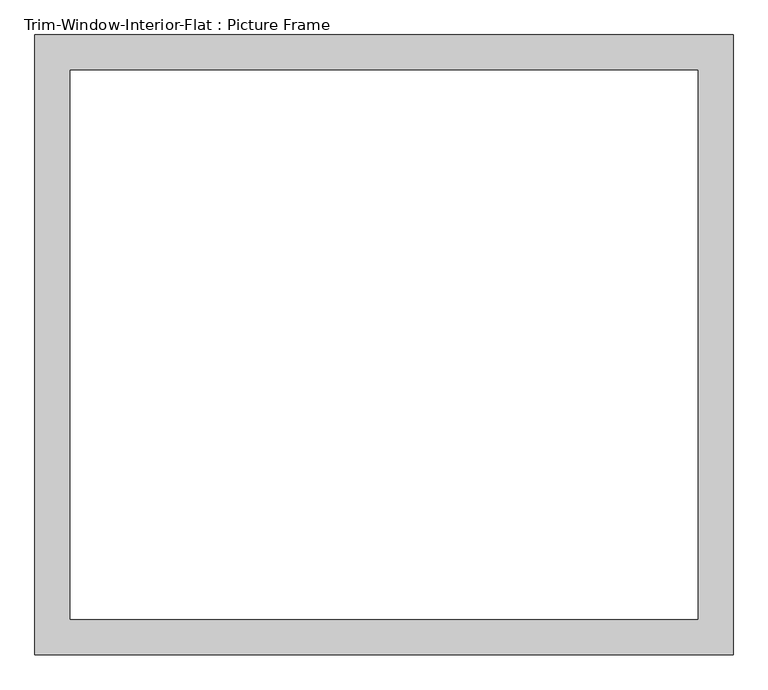
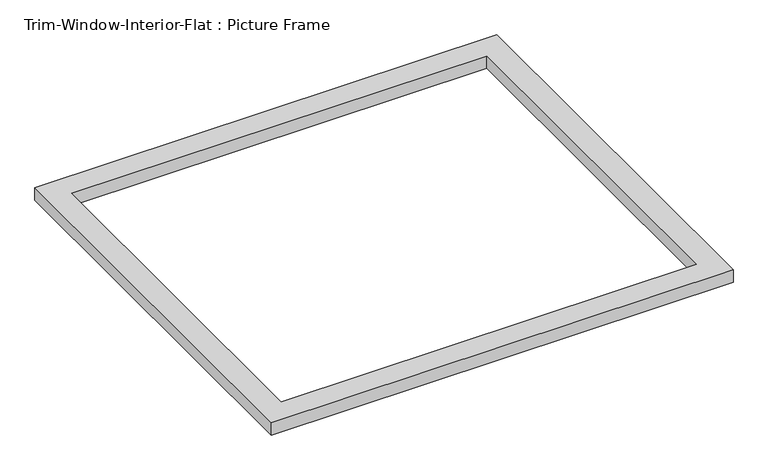
"""IFC4 building model written with IfcOpenShell, lengths in millimetres: proxy geometry, Trim-Window-Interior-Flat : Picture Frame."""

from ifc_helpers import new_model, si_unit, origin, origin_with_axes, place, context, project, spatial, polyline, outline, extrude, source, transform, mapped, element, save


def trim_window_interior_flat_picture_frame_55a9d760(model_context):
    return source(origin(), model_context, "Body", "SweptSolid", [
        extrude(outline(polyline([(565.15, 44.45), (565.15, -958.85), (-565.15, -958.85), (-565.15, 44.45), (565.15, 44.45)]), holes=[polyline([(508.0, -12.7), (-508.0, -12.7), (-508.0, -901.7), (508.0, -901.7), (508.0, -12.7)])]), origin_with_axes(), (0.0, 0.0, 1.0), 31.75),
    ])


if __name__ == "__main__":
    model = new_model("IFC4")
    model_context = context("Model", 3, world=origin())
    ifc_project = project(units=[si_unit("LENGTHUNIT", "METRE", prefix="MILLI")], contexts=[model_context])
    site = spatial("IfcSite", under=ifc_project)
    building = spatial("IfcBuilding", under=site)
    placement = place(None, origin())
    trim_window_interior_flat_picture_frame_shape = trim_window_interior_flat_picture_frame_55a9d760(model_context)
    element("IfcBuildingElementProxy", 1, Name="Trim-Window-Interior-Flat : Picture Frame", ObjectType="Trim-Window-Interior-Flat : Picture Frame", at=placement, inside=building, context=model_context, shape_type="MappedRepresentation", body=[
        mapped(trim_window_interior_flat_picture_frame_shape, transform((0.0, 0.0, 0.0), x_axis=(1.0, 0.0, 0.0), y_axis=(0.0, 1.0, 0.0), z_axis=(0.0, 0.0, 1.0))),
    ])
    save(model, "model.ifc")

# Revit data of these elements
# Type "Trim-Window-Interior-Flat : Picture Frame"
#   Trim Thickness_Picture Frame = 0' - 1 1/4"
#   Trim Width = 0' - 2 1/4"
#   Trim Thickness_with Sill = 0' - 0 3/4"
#   Sill Thickness = 0' - 1 1/4"
#   Opening Width [instance default] = 2' - 0"
#   Opening Height [instance default] = 3' - 0"
#   Default Elevation = 4' - 0"
#   Sill = no
#   Picture Frame = yes
#   Trim Material [instance default] = none
# Element 1 (IfcBuildingElementProxy, "Trim-Window-Interior-Flat : Picture Frame")
#   Opening Width = 3' - 5"
#   Trim Material = Wood - Stained
#   Materials on its faces: "Wood - Stained"
# Materials
#   "Wood - Stained": class "Wood", colour RGB 224 178 126, transparency 0, Cost = 0
